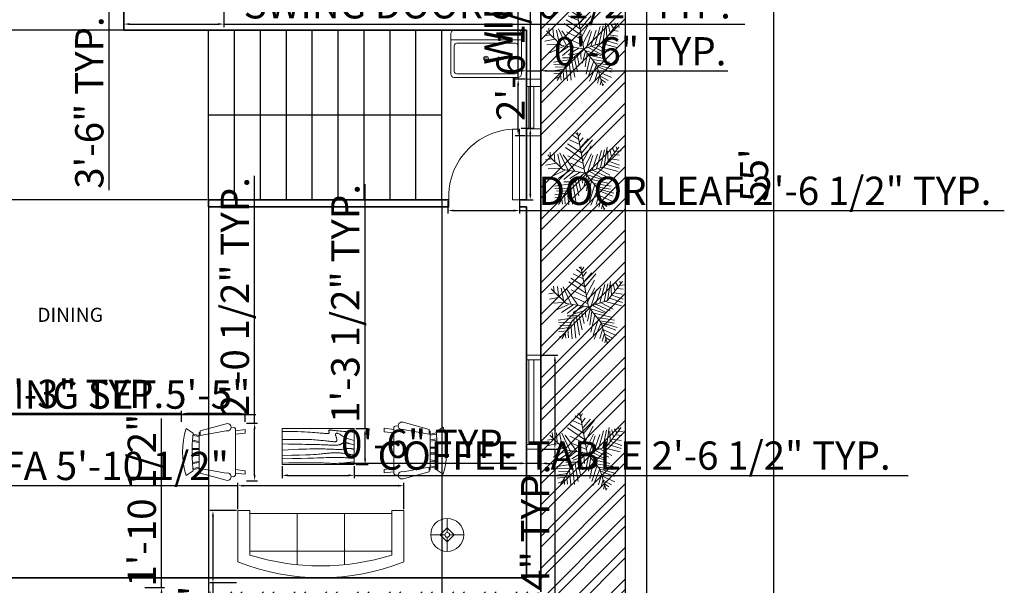
# Model space of a CAD drawing. Units: inches. Extents: x 2297 to 3143, y 440 to 1351.
# Tile 4 of 6: x 2725 to 3143, y 703 to 944. Entities that reach past the tile are written whole.
import ezdxf

# ---------------------------------------------------------------- set-up
doc = ezdxf.new("R2010")
doc.units = ezdxf.units.IN
for name, color, linetype, lineweight in [('A-ANNO-DIMS', 2, 'Continuous', 18), ('A-AREA-IDEN', 7, 'Continuous', 18), ('A-DOOR', 4, 'Continuous', 20), ('A-FLOR-FIXT', 9, 'Continuous', 18), ('A-FLOR-STRS', 7, 'Continuous', 25), ('A-FURN', 8, 'Continuous', 18), ('A-GLAZ', 4, 'Continuous', 18), ('A-WALL', 7, 'Continuous', 35), ('C-PROP', 7, 'Continuous', 25), ('C-SITE-PATT', 252, 'Continuous', 13), ('E-LITE', 9, 'Continuous', 13), ('L-PLNT', 3, 'Continuous', 13)]:
    doc.layers.add(name, color=color, linetype=linetype, lineweight=lineweight)
doc.styles.get("Standard").update_dxf_attribs({"font": 'arial.ttf'})
doc.dimstyles.new('ISO-25', dxfattribs={"dimtxt": 12, "dimasz": 2.5, "dimexe": 1.25, "dimexo": 0.625, "dimtad": 1, "dimdec": 1, "dimlunit": 3, "dimtxsty": 'Standard', "dimcen": 2.5, "dimadec": 0, "dimazin": 0, "dimtfac": 1, "dimtdec": 1, "dimtmove": 0, "dimatfit": 3, "dimfxl": 1, "dimarcsym": 0})

# ---------------------------------------------------------------- blocks, each defined once
blk = doc.blocks.new('Table - Rectangular Woodgrain 60 x 30 in.')
for p, q in [((0, 0), (0, -30)), ((60, 0), (0, 0)), ((60, -30), (60, 0)), ((0, -30), (60, -30))]:
    blk.add_line(p, q)
for points in [[(0, -2.4), (4.8155, -2.418), (9.0302, -2.4688), (12.709, -2.5477), (15.9167, -2.65), (18.7181, -2.7711), (21.1781, -2.9063), (23.3616, -3.0508), (25.3333, -3.2), (27.1477, -3.3495), (28.8172, -3.4958), (30.3437, -3.636), (31.7291, -3.7667), (32.9756, -3.8849), (34.0849, -3.9875), (35.059, -4.0714), (35.9, -4.1334), (36.6114, -4.1711), (37.2041, -4.1854), (37.6906, -4.1779), (38.0833, -4.15), (38.3948, -4.1034), (38.6375, -4.0396), (38.8239, -3.9602), (38.9666, -3.8667), (39.0764, -3.7608), (39.1573, -3.6448), (39.2116, -3.521), (39.2416, -3.3917), (39.2498, -3.2593), (39.2385, -3.1261), (39.21, -2.9944), (39.1666, -2.8667), (39.111, -2.7447), (39.0468, -2.6281), (38.978, -2.5163), (38.9083, -2.4083), (38.8418, -2.3035), (38.7823, -2.201), (38.7337, -2.1001), (38.7, -2), (38.6844, -1.9003), (38.6875, -1.8021), (38.7094, -1.707), (38.75, -1.6167), (38.8094, -1.5326), (38.8875, -1.4563), (38.9844, -1.3893), (39.1, -1.3333), (39.2351, -1.2896), (39.3937, -1.2583), (39.5804, -1.2396), (39.8, -1.2333), (40.057, -1.2396), (40.3562, -1.2583), (40.7023, -1.2896), (41.1, -1.3333), (41.5547, -1.3895), (42.0755, -1.4573), (42.6721, -1.5361), (43.3542, -1.625), (44.1316, -1.7233), (45.014, -1.8302), (46.0114, -1.9449), (47.1333, -2.0667), (48.3862, -2.1947), (49.7625, -2.3281), (51.2513, -2.4663), (52.8416, -2.6083), (54.5226, -2.7535), (56.2833, -2.9011), (58.1127, -3.0501), (60, -3.2)], [(0, -9.2), (6.5759, -9.0858), (11.9385, -9.0365), (16.2527, -9.0418), (19.6833, -9.0917), (22.3952, -9.1759), (24.5531, -9.2844), (26.322, -9.4069), (27.8666, -9.5333), (29.3241, -9.6553), (30.7203, -9.7719), (32.0532, -9.8837), (33.3208, -9.9917), (34.5213, -10.0965), (35.6526, -10.199), (36.7128, -10.2999), (37.7, -10.4), (38.6129, -10.4996), (39.4531, -10.5969), (40.223, -10.6895), (40.925, -10.775), (41.5613, -10.8512), (42.1344, -10.9156), (42.6465, -10.966), (43.1, -11), (43.4976, -11.0158), (43.8437, -11.0136), (44.143, -10.9942), (44.4, -10.9583), (44.6195, -10.9069), (44.8062, -10.8406), (44.9648, -10.7603), (45.1, -10.6667), (45.2155, -10.5598), (45.3114, -10.4365), (45.3871, -10.2929), (45.4416, -10.125), (45.4743, -9.929), (45.4844, -9.7011), (45.4709, -9.4371), (45.4333, -9.1333), (45.3716, -8.7883), (45.2896, -8.4104), (45.1919, -8.0107), (45.0833, -7.6), (44.9685, -7.1893), (44.8521, -6.7896), (44.7388, -6.4117), (44.6333, -6.0667), (44.54, -5.7628), (44.4614, -5.4979), (44.4001, -5.2675), (44.3583, -5.0667), (44.3384, -4.8909), (44.3427, -4.7354), (44.3736, -4.5956), (44.4333, -4.4667), (44.5236, -4.3453), (44.6427, -4.2333), (44.7884, -4.1339), (44.9583, -4.05), (45.1501, -3.9849), (45.3614, -3.9417), (45.59, -3.9234), (45.8333, -3.9333), (46.0915, -3.9749), (46.3734, -4.0531), (46.6906, -4.1736), (47.0542, -4.3417), (47.4756, -4.5629), (47.9661, -4.8427), (48.5372, -5.1866), (49.2, -5.6), (49.9676, -6.0844), (50.8594, -6.625), (51.8965, -7.2031), (53.1, -7.8), (54.491, -8.3969), (56.0906, -8.975), (57.9199, -9.5156), (60, -10)], [(0, -12.8), (5.1847, -12.9322), (9.6213, -13.0323), (13.3963, -13.1059), (16.5958, -13.1583), (19.3063, -13.1952), (21.614, -13.2219), (23.6054, -13.2439), (25.3666, -13.2667), (26.9728, -13.2947), (28.4531, -13.3281), (29.8256, -13.3663), (31.1083, -13.4083), (32.3191, -13.4535), (33.476, -13.501), (34.597, -13.5501), (35.7, -13.6), (36.7984, -13.6497), (37.8875, -13.6979), (38.9578, -13.743), (40, -13.7833), (41.0047, -13.8174), (41.9625, -13.8438), (42.864, -13.8607), (43.7, -13.8667), (44.4631, -13.8604), (45.1552, -13.8417), (45.7801, -13.8104), (46.3416, -13.7667), (46.8439, -13.7104), (47.2906, -13.6417), (47.6858, -13.5604), (48.0333, -13.4667), (48.3375, -13.3608), (48.6042, -13.2448), (48.8396, -13.121), (49.05, -12.9917), (49.2417, -12.8593), (49.4208, -12.7261), (49.5937, -12.5944), (49.7667, -12.4667), (49.9452, -12.3451), (50.1323, -12.2313), (50.3303, -12.1268), (50.5416, -12.0333), (50.7686, -11.9524), (51.0135, -11.8854), (51.2788, -11.8341), (51.5666, -11.8), (51.8785, -11.7843), (52.2116, -11.7865), (52.562, -11.8059), (52.926, -11.8417), (53.2998, -11.8931), (53.6795, -11.9594), (54.0614, -12.0397), (54.4416, -12.1333), (54.8223, -12.2401), (55.2293, -12.3625), (55.6942, -12.5037), (56.2489, -12.6667), (56.9251, -12.8547), (57.7545, -13.0708), (58.7689, -13.3182), (60, -13.6)], [(0, -18), (5.124, -17.7273), (9.6609, -17.5057), (13.6705, -17.3303), (17.2125, -17.1958), (20.3467, -17.0973), (23.1328, -17.0297), (25.6307, -16.9878), (27.9, -16.9667), (29.9928, -16.9617), (31.9302, -16.9703), (33.7254, -16.9907), (35.3917, -17.0208), (36.9423, -17.0588), (38.3906, -17.1026), (39.7499, -17.1503), (41.0333, -17.2), (42.2519, -17.2496), (43.4073, -17.2969), (44.4986, -17.3395), (45.525, -17.375), (46.4858, -17.4012), (47.3802, -17.4156), (48.2074, -17.416), (48.9667, -17.4), (49.6583, -17.3662), (50.2872, -17.3167), (50.8595, -17.2547), (51.3812, -17.1833), (51.8584, -17.1057), (52.2971, -17.025), (52.7034, -16.9443), (53.0833, -16.8667), (53.443, -16.7951), (53.789, -16.7313), (54.128, -16.6768), (54.4666, -16.6334), (54.8115, -16.6024), (55.1693, -16.5854), (55.5465, -16.5841), (55.95, -16.6), (56.3828, -16.6337), (56.8346, -16.6823), (57.2915, -16.7418), (57.7396, -16.8084), (58.165, -16.878), (58.5539, -16.9469), (58.8924, -17.0111), (59.1666, -17.0667), (59.3679, -17.1107), (59.5078, -17.1438), (59.6032, -17.1675), (59.6708, -17.1833), (59.7275, -17.193), (59.7901, -17.1979), (59.8753, -17.1998), (60, -17.2)], [(0, -22.4), (8.0098, -22.2501), (14.4094, -22.1011), (19.4168, -21.9535), (23.25, -21.8083), (26.1269, -21.6663), (28.2656, -21.5281), (29.884, -21.3947), (31.2, -21.2667), (32.3967, -21.1448), (33.5172, -21.0292), (34.5697, -20.9198), (35.5625, -20.8167), (36.5037, -20.7198), (37.4015, -20.6292), (38.2642, -20.5448), (39.1, -20.4667), (39.9164, -20.3951), (40.7187, -20.3313), (41.5117, -20.2768), (42.3, -20.2333), (43.0883, -20.2024), (43.8812, -20.1854), (44.6836, -20.1841), (45.5, -20.2), (46.3328, -20.234), (47.1747, -20.2844), (48.0163, -20.3488), (48.8479, -20.425), (49.66, -20.5106), (50.4429, -20.6031), (51.1872, -20.7004), (51.8833, -20.8), (52.5246, -20.8999), (53.1166, -20.9995), (53.6681, -21.0983), (54.1875, -21.1958), (54.6834, -21.2919), (55.1646, -21.3859), (55.6394, -21.4777), (56.1167, -21.5667), (56.6028, -21.6515), (57.0961, -21.7266), (57.5929, -21.7852), (58.0896, -21.8208), (58.5823, -21.8268), (59.0674, -21.7964), (59.5412, -21.723), (60, -21.6)], [(0, -25.2), (8.6355, -25.0504), (15.7026, -24.9031), (21.4049, -24.7606), (25.9458, -24.625), (29.529, -24.4988), (32.3578, -24.3844), (34.6359, -24.284), (36.5667, -24.2), (38.3213, -24.1341), (39.9417, -24.0854), (41.437, -24.0523), (42.8167, -24.0333), (44.0901, -24.0268), (45.2667, -24.0313), (46.3557, -24.0451), (47.3667, -24.0667), (48.309, -24.0947), (49.1928, -24.1287), (50.0284, -24.168), (50.826, -24.2125), (51.5959, -24.2617), (52.3483, -24.3151), (53.0935, -24.3725), (53.8417, -24.4334), (54.6009, -24.497), (55.3699, -24.561), (56.1454, -24.6226), (56.9239, -24.6792), (57.7021, -24.7279), (58.4764, -24.7662), (59.2435, -24.7911), (60, -24.8)], [(0, -28.8), (5.6867, -28.6681), (10.45, -28.5698), (14.407, -28.5012), (17.675, -28.4584), (20.3711, -28.4374), (22.6125, -28.4344), (24.5164, -28.4455), (26.2, -28.4667), (27.762, -28.4947), (29.2276, -28.5281), (30.6033, -28.5663), (31.8958, -28.6084), (33.1118, -28.6535), (34.2578, -28.7011), (35.3405, -28.7501), (36.3666, -28.8), (37.3443, -28.8497), (38.288, -28.8974), (39.2137, -28.9412), (40.1375, -28.9792), (41.0753, -29.0093), (42.0432, -29.0297), (43.0572, -29.0384), (44.1333, -29.0333), (45.2936, -29.0114), (46.5843, -28.9641), (48.0579, -28.8816), (49.7666, -28.7542), (51.7629, -28.5721), (54.0989, -28.3255), (56.8272, -28.0048), (60, -27.6)]]:
    blk.add_lwpolyline(points)
blk = doc.blocks.new('Sofa - Roundback 7 ft.')
for p, q in [((-12.00002, -32.4421), (-12.00003, -6.5971)), ((11.99997, -32.4421), (11.99998, -6.5971)), ((-36.000027, -34), (-36.000027, -11.4696)), ((-35.999844, -13.3819), (35.9998, -13.3819)), ((35.99998, -34), (35.99998, -11.4696)), ((-36.000027, -32.4421), (35.99998, -32.4421))]:
    blk.add_line(p, q)
for points in [[(-36.000027, -34), (-42.000027, -34), (-42.000027, -8)], [(41.99998, -8), (41.99998, -34), (35.99998, -34)]]:
    blk.add_lwpolyline(points)
for centre, radius, start, end in [((0, -114.25), 114.25, 68.43141, 111.5686), ((-0.00001, -127.1968), 121.1968, 72.72033, 107.2797)]:
    blk.add_arc(centre, radius, start, end)
blk = doc.blocks.new('Chair - Rocking')
for p, q in [((-8, -4.5), (-10, -1.5)), ((-4, -7), (-4.40532, -4.16272)), ((-1.5, -4.05012), (-1.5, -7)), ((-1, -7), (-1, -4.05012)), ((1, -7), (1, -4.04655)), ((1.5, -4.05012), (1.5, -7)), ((8, -4.5), (10, -1.5)), ((-9, -7.5), (-12, -18.49999)), ((-7, -7.5), (-9, -7.5)), ((-9, -18.49999), (-7, -7.5)), ((-8.23428, -6.99939), (-8.3093, -7.47958)), ((-8.23041, -7), (8.23915, -7)), ((-7.5, -4.5), (-7, -7)), ((-6.5, -7), (-7.02225, -4.43)), ((-4.5, -7), (-4.96674, -4.19951)), ((4, -7), (4.40187, -4.18694)), ((4.5, -7), (4.96761, -4.19437)), ((6.5, -7), (7, -4.4057)), ((7.5, -4.5), (7, -7)), ((7, -7.5), (9, -7.5)), ((9, -18.49999), (7, -7.5)), ((8.31071, -7.48854), (8.23449, -7.00073)), ((9, -7.5), (12, -18.49999)), ((-10.36644, -20.64523), (-10.5, -21.49999)), ((10.5, -21.49999), (10.3575, -20.58798)), ((-9, -22.49999), (-9.5, -26.49999)), ((0, -22.49999), (-9.5, -22.49999)), ((-8, -26.49999), (-7.5, -22.49999)), ((0, -22.49999), (9.5, -22.49999)), ((8, -26.49999), (7.5, -22.49999)), ((9, -22.49999), (9.5, -26.49999)), ((-9.5, -26.49999), (-8, -26.49999)), ((9.5, -26.49999), (8, -26.49999))]:
    blk.add_line(p, q)
for centre, radius, start, end in [((0, -34.08333), 34.08333, 72.93847, 107.0615), ((0, -68.25004), 64.25, 93.92211, 97.15267), ((0, -68.25004), 64.25, 82.84733, 93.92211), ((-10.5, -18.99999), 1.58114, 161.5651, 18.43495), ((10.5, -18.99999), 1.58114, 161.5651, 18.43495), ((-9.5, -21.49999), 1, 180, 270), ((9.5, -21.49999), 1, 270, 0)]:
    blk.add_arc(centre, radius, start, end)
blk = doc.blocks.new('Sink-single - 30 in top')
blk.add_line((-15, -3.999996), (15, -3.999996))
for points in [[(-13.5, 0), (13.5, 0)], [(-15, -18.499996), (-15, -1.5)], [(15, -1.5), (15, -18.499996)], [(-13.5, -17.499996), (-13.5, -6.499996)], [(-12.5, -5.499996), (12.5, -5.499996)], [(13.5, -6.499996), (13.5, -17.499996)], [(13.5, -19.999996), (-13.5, -19.999996)], [(12.5, -18.499996), (-12.5, -18.499996)]]:
    blk.add_lwpolyline(points)
for radius in [1, 0.5]:
    blk.add_circle((0, -11.999996), radius)
for centre, radius, start, end in [((-13.5, -1.5), 1.5, 90, 180), ((13.5, -1.5), 1.5, 0, 90), ((-12.5, -6.499996), 1, 90, 180), ((12.5, -6.499996), 1, 0, 90), ((-13.5, -18.499996), 1.5, 180, 270), ((-12.5, -17.499996), 1, 180, 270), ((12.5, -17.499996), 1, 270, 0), ((13.5, -18.499996), 1.5, 270, 0)]:
    blk.add_arc(centre, radius, start, end)
blk = doc.blocks.new('*U16')
for p, q in [((-10.186, 53.64), (-13.084, 55.962)), ((0, 0), (-10.5, 57)), ((-9.099, 51.782), (-6.563, 55.962)), ((-7.288, 39.707), (-21.778, 46.673)), ((-8.737, 47.138), (-17.069, 52.711)), ((-7.65, 43.423), (-2.578, 49.46)), ((-5.839, 35.992), (4.667, 48.067)), ((-5.114, 27.632), (10.463, 46.673)), ((-48.585, 21.131), (-49.309, 29.026)), ((-43.513, 28.561), (-42.427, 15.558)), ((-35.544, 28.097), (-24.314, 3.947)), ((-3.665, 19.273), (-27.574, 35.527)), ((-5.114, 28.097), (-24.676, 40.636)), ((-2.941, 16.486), (8.652, 37.85)), ((16.259, 5.805), (23.142, 31.348)), ((22.055, 7.198), (27.489, 32.277)), ((27, 9), (48, 36)), ((27.127, 9.056), (31.112, 35.992)), ((31.836, 30.883), (32.561, 16.486)), ((35.096, 32.741), (37.27, 22.524)), ((38.719, 34.134), (41.979, 28.561)), ((43.791, 29.954), (51.036, 30.883)), ((44.153, 36.456), (45.239, 32.741)), ((-47.498, 19.737), (-55.83, 18.344)), ((-31.5, 4.5), (-52.5, 25.5)), ((-38.442, 26.239), (-34.819, 7.663)), ((-14.533, 2.09), (-30.834, 25.31)), ((-24.314, 23.917), (-2.941, 13.7)), ((-1.129, 6.734), (9.014, 26.704)), ((3.942, 1.625), (11.187, 24.381)), ((10.101, 3.483), (17.708, 26.239)), ((33.285, 16.486), (48.862, 10.913)), ((36.183, 19.737), (48.137, 17.88)), ((40.53, 25.775), (48.862, 24.846)), ((-40.615, 13.7), (-55.105, 10.913)), ((-33.37, 6.269), (-52.207, 5.34)), ((-28.299, 3.483), (-47.86, -5.805)), ((-21.416, 3.018), (-38.079, -8.128)), ((0, 0), (-31.5, 4.5)), ((-15.982, 2.09), (-30.11, -9.521)), ((0, 0), (-22.5, -19.5)), ((-6.563, 1.161), (-21.416, -8.128)), ((-20.691, 13.7), (-1.129, 4.876)), ((0, 0), (27, 9)), ((0, 0), (18, -22.5)), ((6.478, 1.625), (26.04, -8.592)), ((11.187, 3.483), (30.749, -5.805)), ((18.07, 5.805), (35.096, -3.483)), ((24.229, 7.663), (46.688, 1.625)), ((29.662, 12.307), (48.137, 6.269)), ((-15.257, -12.772), (-30.11, -12.772)), ((-6.563, -5.805), (-19.967, -9.985)), ((-13.446, -11.378), (-8.737, -32.741)), ((-9.461, -8.592), (-6.201, -23.453)), ((-4.752, -3.483), (-3.665, -14.629)), ((2.493, -3.019), (-1.491, -20.202)), ((1.769, -2.555), (24.229, -9.521)), ((5.029, -6.27), (2.131, -25.775)), ((9.014, -11.378), (3.58, -35.992)), ((7.565, -9.056), (32.198, -14.629)), ((-17.431, -15.094), (-42.789, -18.809)), ((-24.314, -21.596), (-42.427, -22.06)), ((-26.849, -26.24), (-40.253, -25.775)), ((-22.5, -19.5), (-37.5, -45)), ((-25.038, -23.918), (-22.865, -45.281)), ((-20.691, -18.345), (-17.793, -44.352)), ((-17.069, -15.094), (-12.721, -40.172)), ((14.085, -16.951), (6.478, -40.172)), ((18.07, -22.524), (8.289, -45.745)), ((12.274, -15.094), (36.907, -18.809)), ((16.259, -19.738), (36.183, -22.989)), ((18, -22.5), (27, -52.5)), ((18.433, -22.524), (40.53, -29.026)), ((19.157, -25.311), (38.719, -33.206)), ((-28.299, -29.026), (-42.789, -31.348)), ((-30.834, -34.135), (-42.427, -35.528)), ((-34.457, -39.708), (-40.978, -42.494)), ((-32.646, -36.921), (-31.921, -44.352)), ((-29.023, -30.884), (-27.936, -43.887)), ((20.244, -30.419), (15.897, -44.816)), ((22.78, -37.85), (19.519, -48.532)), ((21.331, -32.741), (39.081, -40.636)), ((22.78, -38.314), (34.372, -44.816)), ((24.591, -45.745), (23.142, -50.854)), ((24.591, -43.423), (30.749, -47.603)), ((26.764, -49.925), (28.213, -50.854))]:
    blk.add_line(p, q)
blk = doc.blocks.new('*D18')
at = {"layer": 'A-ANNO-DIMS', "color": 0, "lineweight": -2, "transparency": 16777216}
for p, q in [((2993.8, 1207.63), (3046.74, 1207.63)), ((3045.49, 1205.13), (3045.49, 550.13)), ((2992.32, 547.63), (3046.74, 547.63))]:
    blk.add_line(p, q, dxfattribs=at)
at = {"layer": 'A-ANNO-DIMS', "color": 0, "transparency": 16777216}
for points in [[(3045.07, 1205.13), (3045.91, 1205.13), (3045.49, 1207.63)], [(3045.07, 550.13), (3045.91, 550.13), (3045.49, 547.63)]]:
    blk.add_solid(points, dxfattribs=at)
at = {"layer": 'Defpoints', "color": 0, "transparency": 16777216}
for p in [(2993.18, 1207.63), (2991.69, 547.63), (3045.49, 547.63)]:
    blk.add_point(p, dxfattribs=at)
at = {"layer": 'A-ANNO-DIMS', "color": 0, "transparency": 16777216, "insert": (3038.76, 877.63), "char_height": 12, "attachment_point": 5, "rotation": 90}
blk.add_mtext("55'", dxfattribs=at)
blk = doc.blocks.new('Lamp - Table')
for p, q in [((0, 7), (0, 1)), ((-1, 0), (-7, 0)), ((0, 3), (-3, 0)), ((-3, 0), (0, -3)), ((3, 0), (0, 3)), ((0, -3), (3, 0)), ((1, 0), (7, 0)), ((0, -1), (0, -7))]:
    blk.add_line(p, q)
for radius in [7, 1]:
    blk.add_circle((0, 0), radius)
blk = doc.blocks.new('DOOR-30IN-LEAF')
blk.add_lwpolyline([(30, 0), (27, 0), (27, 30), (30, 30)], close=True)
blk.add_arc((28.5, 1.5), 28.54, 86.9872, 183.0128)
blk = doc.blocks.new('WIN-36IN-6IN-WALL')
for p, q in [((6, 40), (0, 40)), ((6, 38), (0, 38)), ((3, 38), (3, 2)), ((5, 38), (5, 2)), ((0, 2), (6, 2)), ((0, 0), (6, 0))]:
    blk.add_line(p, q)
blk = doc.blocks.new('WIN-18IN-6IN-WALL')
for p, q in [((6, 24), (0, 24)), ((6, 21), (0, 21)), ((1, 3), (1, 21)), ((3, 3), (3, 21)), ((0, 3), (6, 3)), ((0, 0), (6, 0))]:
    blk.add_line(p, q)
blk = doc.blocks.new('*D29')
at = {"layer": 'A-ANNO-DIMS', "color": 0, "lineweight": -2, "transparency": 16777216}
for p, q in [((2769.69, 947.51), (2769.69, 940.52)), ((2812.11, 947.51), (2812.11, 940.52)), ((2772.19, 941.77), (2809.61, 941.77)), ((2812.11, 941.77), (3033.33, 941.77))]:
    blk.add_line(p, q, dxfattribs=at)
at = {"layer": 'A-ANNO-DIMS', "color": 0, "transparency": 16777216}
for points in [[(2772.19, 942.19), (2772.19, 941.35), (2769.69, 941.77)], [(2809.61, 942.19), (2809.61, 941.35), (2812.11, 941.77)]]:
    blk.add_solid(points, dxfattribs=at)
at = {"layer": 'Defpoints', "color": 0, "transparency": 16777216}
for p in [(2769.69, 948.13), (2812.11, 948.13), (2812.11, 941.77)]:
    blk.add_point(p, dxfattribs=at)
at = {"layer": 'A-ANNO-DIMS', "color": 0, "transparency": 16777216, "insert": (2923.97, 948.61), "char_height": 12, "attachment_point": 5}
blk.add_mtext('SWING DOOR 3\'-6 1/2" TYP.', dxfattribs=at)
blk = doc.blocks.new('*D30')
at = {"layer": 'A-ANNO-DIMS', "color": 0, "lineweight": -2, "transparency": 16777216}
for p, q in [((2769.07, 990.13), (2762.08, 990.13)), ((2763.33, 987.63), (2763.33, 950.63)), ((2769.07, 948.13), (2762.08, 948.13)), ((2763.33, 948.13), (2763.33, 871.25))]:
    blk.add_line(p, q, dxfattribs=at)
at = {"layer": 'A-ANNO-DIMS', "color": 0, "transparency": 16777216}
for points in [[(2762.91, 987.63), (2763.75, 987.63), (2763.33, 990.13)], [(2762.91, 950.63), (2763.75, 950.63), (2763.33, 948.13)]]:
    blk.add_solid(points, dxfattribs=at)
at = {"layer": 'Defpoints', "color": 0, "transparency": 16777216}
for p in [(2769.69, 990.13), (2763.33, 948.13), (2769.69, 948.13)]:
    blk.add_point(p, dxfattribs=at)
at = {"layer": 'A-ANNO-DIMS', "color": 0, "transparency": 16777216, "insert": (2756.57, 908.44), "char_height": 12, "attachment_point": 5, "rotation": 90}
blk.add_mtext('3\'-6" TYP.', dxfattribs=at)
blk = doc.blocks.new('*D31')
at = {"layer": 'A-ANNO-DIMS', "color": 0, "lineweight": -2, "transparency": 16777216}
for p, q in [((2947.32, 801.2), (2953.94, 801.2)), ((2952.69, 798.7), (2952.69, 763.7)), ((2947.32, 761.2), (2953.94, 761.2)), ((2952.69, 761.2), (2952.69, 605.6))]:
    blk.add_line(p, q, dxfattribs=at)
at = {"layer": 'A-ANNO-DIMS', "color": 0, "transparency": 16777216}
for points in [[(2952.28, 798.7), (2953.11, 798.7), (2952.69, 801.2)], [(2952.28, 763.7), (2953.11, 763.7), (2952.69, 761.2)]]:
    blk.add_solid(points, dxfattribs=at)
at = {"layer": 'Defpoints', "color": 0, "transparency": 16777216}
for p in [(2946.69, 801.2), (2946.69, 761.2), (2952.69, 761.2)]:
    blk.add_point(p, dxfattribs=at)
at = {"layer": 'A-ANNO-DIMS', "color": 0, "transparency": 16777216, "insert": (2945.85, 682.15), "char_height": 12, "attachment_point": 5, "rotation": 90}
blk.add_mtext('WINDOW 3\'-4" TYP.', dxfattribs=at)
blk = doc.blocks.new('*D32')
at = {"layer": 'A-ANNO-DIMS', "color": 0, "lineweight": -2, "transparency": 16777216}
for p, q in [((2940.69, 760.58), (2940.69, 753.95)), ((2946.69, 760.58), (2946.69, 753.95)), ((2938.19, 755.2), (2861.3, 755.2)), ((2946.69, 755.2), (2940.69, 755.2)), ((2949.19, 755.2), (2951.69, 755.2))]:
    blk.add_line(p, q, dxfattribs=at)
at = {"layer": 'A-ANNO-DIMS', "color": 0, "transparency": 16777216}
for points in [[(2938.19, 755.62), (2938.19, 754.78), (2940.69, 755.2)], [(2949.19, 755.62), (2949.19, 754.78), (2946.69, 755.2)]]:
    blk.add_solid(points, dxfattribs=at)
at = {"layer": 'Defpoints', "color": 0, "transparency": 16777216}
for p in [(2940.69, 761.2), (2946.69, 761.2), (2940.69, 755.2)]:
    blk.add_point(p, dxfattribs=at)
at = {"layer": 'A-ANNO-DIMS', "color": 0, "transparency": 16777216, "insert": (2898.49, 761.95), "char_height": 12, "attachment_point": 5}
blk.add_mtext('0\'-6" TYP.', dxfattribs=at)
blk = doc.blocks.new('*D43')
at = {"layer": 'A-ANNO-DIMS', "color": 0, "lineweight": -2, "transparency": 16777216}
for p, q in [((2937.09, 918.32), (2937.09, 1073.92)), ((2940.07, 918.32), (2935.84, 918.32)), ((2937.09, 896.82), (2937.09, 915.82)), ((2940.07, 894.32), (2935.84, 894.32))]:
    blk.add_line(p, q, dxfattribs=at)
at = {"layer": 'A-ANNO-DIMS', "color": 0, "transparency": 16777216}
for points in [[(2936.68, 915.82), (2937.51, 915.82), (2937.09, 918.32)], [(2936.68, 896.82), (2937.51, 896.82), (2937.09, 894.32)]]:
    blk.add_solid(points, dxfattribs=at)
at = {"layer": 'Defpoints', "color": 0, "transparency": 16777216}
for p in [(2937.09, 918.32), (2940.69, 918.32), (2940.69, 894.32)]:
    blk.add_point(p, dxfattribs=at)
at = {"layer": 'A-ANNO-DIMS', "color": 0, "transparency": 16777216, "insert": (2930.26, 997.37), "char_height": 12, "attachment_point": 5, "rotation": 90}
blk.add_mtext('WINDOW 2\'-0" TYP.', dxfattribs=at)
blk = doc.blocks.new('*D44')
at = {"layer": 'A-ANNO-DIMS', "color": 0, "lineweight": -2, "transparency": 16777216}
for p, q in [((2938.19, 921.92), (2935.69, 921.92)), ((2940.69, 918.95), (2940.69, 923.17)), ((2940.69, 921.92), (2946.69, 921.92)), ((2946.69, 918.95), (2946.69, 923.17)), ((2949.19, 921.92), (3026.09, 921.92))]:
    blk.add_line(p, q, dxfattribs=at)
at = {"layer": 'A-ANNO-DIMS', "color": 0, "transparency": 16777216}
for points in [[(2938.19, 922.34), (2938.19, 921.5), (2940.69, 921.92)], [(2949.19, 922.34), (2949.19, 921.5), (2946.69, 921.92)]]:
    blk.add_solid(points, dxfattribs=at)
at = {"layer": 'Defpoints', "color": 0, "transparency": 16777216}
for p in [(2946.69, 921.92), (2940.69, 918.32), (2946.69, 918.32)]:
    blk.add_point(p, dxfattribs=at)
at = {"layer": 'A-ANNO-DIMS', "color": 0, "transparency": 16777216, "insert": (2988.89, 928.67), "char_height": 12, "attachment_point": 5}
blk.add_mtext('0\'-6" TYP.', dxfattribs=at)
blk = doc.blocks.new('*D45')
at = {"layer": 'A-ANNO-DIMS', "color": 0, "lineweight": -2, "transparency": 16777216}
for p, q in [((2836.9, 754.07), (2836.9, 748.85)), ((2867.52, 754.07), (2867.52, 748.85)), ((2839.4, 750.1), (2865.02, 750.1)), ((2867.52, 750.1), (3102.65, 750.1))]:
    blk.add_line(p, q, dxfattribs=at)
at = {"layer": 'A-ANNO-DIMS', "color": 0, "transparency": 16777216}
for points in [[(2839.4, 750.52), (2839.4, 749.69), (2836.9, 750.1)], [(2865.02, 750.52), (2865.02, 749.69), (2867.52, 750.1)]]:
    blk.add_solid(points, dxfattribs=at)
at = {"layer": 'Defpoints', "color": 0, "transparency": 16777216}
for p in [(2836.9, 754.69), (2867.52, 754.69), (2867.52, 750.1)]:
    blk.add_point(p, dxfattribs=at)
at = {"layer": 'A-ANNO-DIMS', "color": 0, "transparency": 16777216, "insert": (2986.33, 756.94), "char_height": 12, "attachment_point": 5}
blk.add_mtext('COFFEE TABLE 2\'-6 1/2" TYP.', dxfattribs=at)
blk = doc.blocks.new('*D46')
at = {"layer": 'A-ANNO-DIMS', "color": 0, "lineweight": -2, "transparency": 16777216}
for p, q in [((2872.11, 770), (2872.11, 873.73)), ((2868.14, 770), (2873.36, 770)), ((2872.11, 757.19), (2872.11, 767.5)), ((2868.14, 754.69), (2873.36, 754.69))]:
    blk.add_line(p, q, dxfattribs=at)
at = {"layer": 'A-ANNO-DIMS', "color": 0, "transparency": 16777216}
for points in [[(2871.69, 767.5), (2872.53, 767.5), (2872.11, 770)], [(2871.69, 757.19), (2872.53, 757.19), (2872.11, 754.69)]]:
    blk.add_solid(points, dxfattribs=at)
at = {"layer": 'Defpoints', "color": 0, "transparency": 16777216}
for p in [(2867.52, 770), (2872.11, 770), (2867.52, 754.69)]:
    blk.add_point(p, dxfattribs=at)
at = {"layer": 'A-ANNO-DIMS', "color": 0, "transparency": 16777216, "insert": (2865.27, 823.11), "char_height": 12, "attachment_point": 5, "rotation": 90}
blk.add_mtext('1\'-3 1/2" TYP.', dxfattribs=at)
blk = doc.blocks.new('*D48')
at = {"layer": 'A-ANNO-DIMS', "color": 0, "lineweight": -2, "transparency": 16777216}
for p, q in [((2778.39, 676.96), (2778.39, 683.36)), ((2780.89, 682.11), (2799.4, 682.11)), ((2801.9, 676.96), (2801.9, 683.36)), ((2801.9, 682.11), (2914.95, 682.11))]:
    blk.add_line(p, q, dxfattribs=at)
at = {"layer": 'A-ANNO-DIMS', "color": 0, "transparency": 16777216}
for points in [[(2780.89, 682.52), (2780.89, 681.69), (2778.39, 682.11)], [(2799.4, 682.52), (2799.4, 681.69), (2801.9, 682.11)]]:
    blk.add_solid(points, dxfattribs=at)
at = {"layer": 'Defpoints', "color": 0, "transparency": 16777216}
for p in [(2801.9, 682.11), (2778.39, 676.34), (2801.9, 676.34)]:
    blk.add_point(p, dxfattribs=at)
at = {"layer": 'A-ANNO-DIMS', "color": 0, "transparency": 16777216, "insert": (2859.68, 688.94), "char_height": 12, "attachment_point": 5}
blk.add_mtext('1\'-11 1/2" TYP.', dxfattribs=at)
blk = doc.blocks.new('*D49')
at = {"layer": 'A-ANNO-DIMS', "color": 0, "lineweight": -2, "transparency": 16777216}
for p, q in [((2818.08, 745.72), (2694.9, 745.72)), ((2818.08, 735.78), (2818.08, 746.97)), ((2886.03, 745.72), (2820.58, 745.72)), ((2888.53, 735.78), (2888.53, 746.97))]:
    blk.add_line(p, q, dxfattribs=at)
at = {"layer": 'A-ANNO-DIMS', "color": 0, "transparency": 16777216}
for points in [[(2820.58, 746.14), (2820.58, 745.3), (2818.08, 745.72)], [(2886.03, 746.14), (2886.03, 745.3), (2888.53, 745.72)]]:
    blk.add_solid(points, dxfattribs=at)
at = {"layer": 'Defpoints', "color": 0, "transparency": 16777216}
for p in [(2818.08, 745.72), (2818.08, 735.15), (2888.53, 735.15)]:
    blk.add_point(p, dxfattribs=at)
at = {"layer": 'A-ANNO-DIMS', "color": 0, "transparency": 16777216, "insert": (2755.24, 752.55), "char_height": 12, "attachment_point": 5}
blk.add_mtext('SOFA 5\'-10 1/2"', dxfattribs=at)
blk = doc.blocks.new('*D50')
at = {"layer": 'A-ANNO-DIMS', "color": 0, "lineweight": -2, "transparency": 16777216}
for p, q in [((2817.45, 735.15), (2806.26, 735.15)), ((2807.51, 732.65), (2807.51, 706.9)), ((2817.45, 704.4), (2806.26, 704.4)), ((2807.51, 704.4), (2807.51, 668.54))]:
    blk.add_line(p, q, dxfattribs=at)
at = {"layer": 'A-ANNO-DIMS', "color": 0, "transparency": 16777216}
for points in [[(2807.09, 732.65), (2807.92, 732.65), (2807.51, 735.15)], [(2807.09, 706.9), (2807.92, 706.9), (2807.51, 704.4)]]:
    blk.add_solid(points, dxfattribs=at)
at = {"layer": 'Defpoints', "color": 0, "transparency": 16777216}
for p in [(2818.08, 735.15), (2807.51, 704.4), (2818.08, 704.4)]:
    blk.add_point(p, dxfattribs=at)
at = {"layer": 'A-ANNO-DIMS', "color": 0, "transparency": 16777216, "insert": (2800.86, 685.22), "char_height": 12, "attachment_point": 5, "rotation": 90}
blk.add_mtext('2\'-7"', dxfattribs=at)
blk = doc.blocks.new('*D52')
at = {"layer": 'A-ANNO-DIMS', "color": 0, "lineweight": -2, "transparency": 16777216}
for p, q in [((2785.68, 702.41), (2785.68, 774.21)), ((2778.53, 702.41), (2786.93, 702.41)), ((2785.68, 682.29), (2785.68, 699.91)), ((2778.53, 679.79), (2786.93, 679.79))]:
    blk.add_line(p, q, dxfattribs=at)
at = {"layer": 'A-ANNO-DIMS', "color": 0, "transparency": 16777216}
for points in [[(2785.26, 699.91), (2786.09, 699.91), (2785.68, 702.41)], [(2785.26, 682.29), (2786.09, 682.29), (2785.68, 679.79)]]:
    blk.add_solid(points, dxfattribs=at)
at = {"layer": 'Defpoints', "color": 0, "transparency": 16777216}
for p in [(2777.91, 702.41), (2785.68, 702.41), (2777.91, 679.79)]:
    blk.add_point(p, dxfattribs=at)
at = {"layer": 'A-ANNO-DIMS', "color": 0, "transparency": 16777216, "insert": (2778.85, 739.56), "char_height": 12, "attachment_point": 5, "rotation": 90}
blk.add_mtext('1\'-10 1/2"', dxfattribs=at)
blk = doc.blocks.new('*D53')
at = {"layer": 'A-ANNO-DIMS', "color": 0, "lineweight": -2, "transparency": 16777216}
for p, q in [((2794.15, 772.88), (2794.15, 777.56)), ((2821.15, 772.88), (2821.15, 777.56)), ((2794.15, 776.31), (2641.5, 776.31)), ((2818.65, 776.31), (2796.65, 776.31))]:
    blk.add_line(p, q, dxfattribs=at)
at = {"layer": 'A-ANNO-DIMS', "color": 0, "transparency": 16777216}
for points in [[(2796.65, 776.72), (2796.65, 775.89), (2794.15, 776.31)], [(2818.65, 776.72), (2818.65, 775.89), (2821.15, 776.31)]]:
    blk.add_solid(points, dxfattribs=at)
at = {"layer": 'Defpoints', "color": 0, "transparency": 16777216}
for p in [(2794.15, 776.31), (2794.15, 772.26), (2821.15, 772.26)]:
    blk.add_point(p, dxfattribs=at)
at = {"layer": 'A-ANNO-DIMS', "color": 0, "transparency": 16777216, "insert": (2716.58, 783.14), "char_height": 12, "attachment_point": 5}
blk.add_mtext('ROCKER 2\'-3" TYP.', dxfattribs=at)
blk = doc.blocks.new('*D54')
at = {"layer": 'A-ANNO-DIMS', "color": 0, "lineweight": -2, "transparency": 16777216}
for p, q in [((2825.2, 772.26), (2825.2, 877.32)), ((2821.78, 772.26), (2826.45, 772.26)), ((2825.2, 750.32), (2825.2, 769.76)), ((2821.78, 747.82), (2826.45, 747.82))]:
    blk.add_line(p, q, dxfattribs=at)
at = {"layer": 'A-ANNO-DIMS', "color": 0, "transparency": 16777216}
for points in [[(2824.79, 769.76), (2825.62, 769.76), (2825.2, 772.26)], [(2824.79, 750.32), (2825.62, 750.32), (2825.2, 747.82)]]:
    blk.add_solid(points, dxfattribs=at)
at = {"layer": 'Defpoints', "color": 0, "transparency": 16777216}
for p in [(2821.15, 772.26), (2825.2, 772.26), (2821.15, 747.82)]:
    blk.add_point(p, dxfattribs=at)
at = {"layer": 'A-ANNO-DIMS', "color": 0, "transparency": 16777216, "insert": (2818.37, 826.04), "char_height": 12, "attachment_point": 5, "rotation": 90}
blk.add_mtext('2\'-0 1/2" TYP.', dxfattribs=at)
blk = doc.blocks.new('*D57')
at = {"layer": 'A-ANNO-DIMS', "color": 0, "lineweight": -2, "transparency": 16777216}
for p, q in [((2907.27, 866.51), (2907.27, 861.32)), ((2937.69, 866.51), (2937.69, 861.32)), ((2909.77, 862.57), (2935.19, 862.57)), ((2937.69, 862.57), (3143.49, 862.57))]:
    blk.add_line(p, q, dxfattribs=at)
at = {"layer": 'A-ANNO-DIMS', "color": 0, "transparency": 16777216}
for points in [[(2909.77, 862.99), (2909.77, 862.15), (2907.27, 862.57)], [(2935.19, 862.99), (2935.19, 862.15), (2937.69, 862.57)]]:
    blk.add_solid(points, dxfattribs=at)
at = {"layer": 'Defpoints', "color": 0, "transparency": 16777216}
for p in [(2907.27, 867.13), (2937.69, 867.13), (2937.69, 862.57)]:
    blk.add_point(p, dxfattribs=at)
at = {"layer": 'A-ANNO-DIMS', "color": 0, "transparency": 16777216, "insert": (3041.84, 869.4), "char_height": 12, "attachment_point": 5}
blk.add_mtext('DOOR LEAF 2\'-6 1/2" TYP.', dxfattribs=at)
blk = doc.blocks.new('*D58')
at = {"layer": 'A-ANNO-DIMS', "color": 0, "lineweight": -2, "transparency": 16777216}
for p, q in [((2942.26, 897.56), (2942.26, 1002.62)), ((2938.32, 897.56), (2943.51, 897.56)), ((2942.26, 869.63), (2942.26, 895.06)), ((2938.32, 867.13), (2943.51, 867.13))]:
    blk.add_line(p, q, dxfattribs=at)
at = {"layer": 'A-ANNO-DIMS', "color": 0, "transparency": 16777216}
for points in [[(2941.84, 895.06), (2942.67, 895.06), (2942.26, 897.56)], [(2941.84, 869.63), (2942.67, 869.63), (2942.26, 867.13)]]:
    blk.add_solid(points, dxfattribs=at)
at = {"layer": 'Defpoints', "color": 0, "transparency": 16777216}
for p in [(2937.69, 897.56), (2942.26, 897.56), (2937.69, 867.13)]:
    blk.add_point(p, dxfattribs=at)
at = {"layer": 'A-ANNO-DIMS', "color": 0, "transparency": 16777216, "insert": (2935.43, 951.34), "char_height": 12, "attachment_point": 5, "rotation": 90}
blk.add_mtext('2\'-6 1/2" TYP.', dxfattribs=at)
blk = doc.blocks.new('*D63')
at = {"layer": 'A-ANNO-DIMS', "color": 0, "lineweight": -2, "transparency": 16777216}
for p, q in [((2625.28, 785.11), (2625.28, 774.77)), ((2690.07, 785.11), (2690.07, 774.77)), ((2627.78, 776.02), (2687.57, 776.02)), ((2690.07, 776.02), (2825.72, 776.02))]:
    blk.add_line(p, q, dxfattribs=at)
at = {"layer": 'A-ANNO-DIMS', "color": 0, "transparency": 16777216}
for points in [[(2627.78, 776.44), (2627.78, 775.6), (2625.28, 776.02)], [(2687.57, 776.44), (2687.57, 775.6), (2690.07, 776.02)]]:
    blk.add_solid(points, dxfattribs=at)
at = {"layer": 'Defpoints', "color": 0, "transparency": 16777216}
for p in [(2625.28, 785.74), (2690.07, 785.74), (2690.07, 776.02)]:
    blk.add_point(p, dxfattribs=at)
at = {"layer": 'A-ANNO-DIMS', "color": 0, "transparency": 16777216, "insert": (2759.14, 782.85), "char_height": 12, "attachment_point": 5}
blk.add_mtext('DINING SET 5\'-5"', dxfattribs=at)
blk = doc.blocks.new('*D79')
at = {"layer": 'A-ANNO-DIMS', "color": 0, "lineweight": -2, "transparency": 16777216}
for p, q in [((2805.69, 866.51), (2805.69, 510.33)), ((2904.69, 866.51), (2904.69, 510.33)), ((2808.19, 511.58), (2902.19, 511.58))]:
    blk.add_line(p, q, dxfattribs=at)
at = {"layer": 'A-ANNO-DIMS', "color": 0, "transparency": 16777216}
for points in [[(2808.19, 512), (2808.19, 511.17), (2805.69, 511.58)], [(2902.19, 512), (2902.19, 511.17), (2904.69, 511.58)]]:
    blk.add_solid(points, dxfattribs=at)
at = {"layer": 'Defpoints', "color": 0, "transparency": 16777216}
for p in [(2805.69, 867.13), (2904.69, 867.13), (2904.69, 511.58)]:
    blk.add_point(p, dxfattribs=at)
at = {"layer": 'A-ANNO-DIMS', "color": 0, "transparency": 16777216, "insert": (2855.19, 518.34), "char_height": 12, "attachment_point": 5}
blk.add_mtext('8\'-3"', dxfattribs=at)
blk = doc.blocks.new('*D80')
at = {"layer": 'A-ANNO-DIMS', "color": 0, "lineweight": -2, "transparency": 16777216}
for p, q in [((2805.07, 939.13), (2355.89, 939.13)), ((2357.14, 869.63), (2357.14, 936.63)), ((2805.07, 867.13), (2355.89, 867.13))]:
    blk.add_line(p, q, dxfattribs=at)
at = {"layer": 'A-ANNO-DIMS', "color": 0, "transparency": 16777216}
for points in [[(2356.73, 936.63), (2357.56, 936.63), (2357.14, 939.13)], [(2356.73, 869.63), (2357.56, 869.63), (2357.14, 867.13)]]:
    blk.add_solid(points, dxfattribs=at)
at = {"layer": 'Defpoints', "color": 0, "transparency": 16777216}
for p in [(2357.14, 939.13), (2805.69, 939.13), (2805.69, 867.13)]:
    blk.add_point(p, dxfattribs=at)
at = {"layer": 'A-ANNO-DIMS', "color": 0, "transparency": 16777216, "insert": (2350.39, 903.13), "char_height": 12, "attachment_point": 5, "rotation": 90}
blk.add_mtext('6\'-0"', dxfattribs=at)

msp = doc.modelspace()

# ---------------------------------------------------------------- hatches: boundary and pattern name
at = {"layer": 'C-SITE-PATT'}
h = msp.add_hatch(dxfattribs=at)
h.set_pattern_fill('ANSI32', color=256)
h.paths.add_polyline_path([(2438.19, 1198.63), (2402.19, 1198.63), (2402.19, 556.63), (2667.43, 556.63), (2742.43, 556.63), (2946.69, 556.63), (2982.69, 556.63), (2982.69, 1117.63), (2982.69, 1123.63), (2982.69, 1198.63), (2946.69, 1198.63), (2946.69, 1117.63), (2946.69, 700.63), (2806.19, 700.63), (2806.19, 580.63), (2738.57, 580.63), (2738.57, 589.63), (2735.57, 589.63), (2735.57, 625.63, 0.402069), (2702.6, 591.13, 0.401544), (2669.57, 625.63), (2669.57, 589.63), (2666.57, 589.63), (2666.57, 580.63), (2438.19, 580.63)])
h.paths.add_polyline_path([(2706.46, 558.2, -0.000472), (2706.46, 558.13, -0.000473)], flags=16)
h.paths.add_polyline_path([(2875.15, 576.11), (2920.92, 576.11), (2920.92, 585.31), (2875.15, 585.31)], flags=24)
h.paths.add_polyline_path([(2875.13, 585.74), (2915.96, 585.74), (2915.96, 595.05), (2875.13, 595.05)], flags=24)
h.paths.add_polyline_path([(2646.52, 1069.72), (2687.63, 1069.72), (2687.63, 1078.92), (2646.52, 1078.92)], flags=25)
h.paths.add_polyline_path([(2646.5, 1079.35), (2686.39, 1079.35), (2686.39, 1088.65), (2646.5, 1088.65)], flags=25)

# ---------------------------------------------------------------- linework, layer by layer
at = {"layer": 'A-DOOR'}
for p, q in [((2904.69, 867.13), (2904.69, 864.13)), ((2907.69, 867.13), (2907.69, 864.13)), ((2937.69, 867.13), (2937.69, 864.13))]:
    msp.add_line(p, q, dxfattribs=at)
at = {"layer": 'A-FLOR-STRS'}
for p, q in [((2805.69, 867.13), (2805.69, 939.13)), ((2816.69, 867.13), (2816.69, 939.13)), ((2827.69, 867.13), (2827.69, 939.13)), ((2838.69, 867.13), (2838.69, 939.13)), ((2849.69, 867.13), (2849.69, 939.13)), ((2860.69, 867.13), (2860.69, 939.13)), ((2871.69, 867.13), (2871.69, 939.13)), ((2882.69, 867.13), (2882.69, 939.13)), ((2893.69, 867.13), (2893.69, 939.13)), ((2904.69, 867.13), (2904.69, 939.13)), ((2904.69, 903.13), (2805.69, 903.13))]:
    msp.add_line(p, q, dxfattribs=at)
at = {"layer": 'A-WALL'}
for p, q in [((2946.69, 700.63), (2946.69, 1117.63)), ((2769.69, 939.13), (2769.69, 951.13)), ((2940.69, 939.13), (2769.69, 939.13)), ((2940.69, 867.13), (2940.69, 939.13)), ((2805.69, 867.13), (2805.69, 864.13)), ((2907.69, 867.13), (2805.69, 867.13)), ((2940.69, 867.13), (2937.69, 867.13)), ((2907.69, 864.13), (2805.69, 864.13)), ((2940.69, 864.13), (2937.69, 864.13)), ((2940.69, 706.63), (2940.69, 864.13)), ((2642.19, 706.63), (2940.69, 706.63))]:
    msp.add_line(p, q, dxfattribs=at)
at = {"layer": 'C-PROP'}
msp.add_line((2982.69, 556.63), (2982.69, 1117.63), dxfattribs=at)
msp.add_lwpolyline([(2742.43, 547.63), (2991.69, 547.63), (2991.69, 1207.63), (2393.19, 1207.63)], dxfattribs=at)

# ---------------------------------------------------------------- block references
at = {"layer": 'A-DOOR'}
msp.add_blockref('DOOR-30IN-LEAF', (2907.69, 867.13), dxfattribs=at)
at = {"layer": 'A-FLOR-FIXT'}
msp.add_blockref('Sink-single - 30 in top', (2923.49, 939.13), dxfattribs=at)
at = {"layer": 'A-FURN'}
for p, rotation in [((2794.65, 760.04), 90), ((2906.76, 760.64), 270)]:
    msp.add_blockref('Chair - Rocking', p, dxfattribs=dict(at, rotation=rotation))
at = {"layer": 'A-FURN', "xscale": 0.5102167871031984, "yscale": 0.5102167871031984, "zscale": 0.5102167871031984}
msp.add_blockref('Table - Rectangular Woodgrain 60 x 30 in.', (2836.9, 770), dxfattribs=at)
at = {"layer": 'A-FURN', "xscale": 0.8387243295483651, "yscale": 0.8387243295483651, "zscale": 0.8387243295483651, "rotation": 180}
msp.add_blockref('Sofa - Roundback 7 ft.', (2853.3, 706.63), dxfattribs=at)
at = {"layer": 'A-GLAZ'}
msp.add_blockref('WIN-18IN-6IN-WALL', (2940.69, 894.32), dxfattribs=at)
at = {"layer": 'A-GLAZ', "rotation": 180}
msp.add_blockref('WIN-36IN-6IN-WALL', (2946.69, 801.2), dxfattribs=at)
at = {"layer": 'E-LITE'}
msp.add_blockref('Lamp - Table', (2906.96, 724.83), dxfattribs=at)
at = {"layer": 'L-PLNT', "xscale": 0.3005060358918508, "yscale": 0.3005060358918508, "zscale": 0.3005060358918508}
for p in [(2964.92, 931.29), (2965.46, 878.63), (2966.92, 821.68), (2966.38, 759.56)]:
    msp.add_blockref('*U16', p, dxfattribs=at)

# ---------------------------------------------------------------- texts
at = {"layer": 'A-AREA-IDEN'}
msp.add_text('DINING', height=6, dxfattribs=at).set_placement((2732.92, 815.29))

# ---------------------------------------------------------------- dimensions: what is measured, and where the dimension line sits
at = {"layer": 'A-ANNO-DIMS'}
for base, p1, p2, angle, override, picture, middle in [((3045.49, 547.63), (2993.18, 1207.63), (2991.69, 547.63), 90, {"dimclrd": 0, "dimclre": 0, "dimclrt": 0}, '*D18', (3038.76, 877.63)), ((2357.14, 939.13), (2805.69, 867.13), (2805.69, 939.13), 90, {"dimdec": 1, "dimlfac": 1, "dimrnd": 0, "dimzin": 1, "dimdsep": 46, "dimlunit": 4, "dimfrac": 2}, '*D80', (2350.39, 903.13)), ((2785.68, 702.41), (2777.91, 679.79), (2777.91, 702.41), 90, {"dimdec": 1, "dimlfac": 1, "dimrnd": 0, "dimzin": 1, "dimdsep": 46, "dimlunit": 4, "dimfrac": 2}, '*D52', (2778.85, 739.56)), ((2807.5075, 704.3978), (2818.0754, 735.151), (2818.0754, 704.3978), 270, {"dimdec": 1, "dimlfac": 1, "dimrnd": 0, "dimzin": 1, "dimdsep": 46, "dimlunit": 4, "dimfrac": 2}, '*D50', (2800.8579, 685.221))]:
    dim = msp.add_linear_dim(base=base, p1=p1, p2=p2, angle=angle, dimstyle='ISO-25', override=override, dxfattribs=at)
    dim.commit()
    dim.dimension.update_dxf_attribs({"geometry": picture, "text_midpoint": middle})
for base, p1, p2, angle, text, picture, middle in [((2937.09, 918.32), (2940.69, 894.32), (2940.69, 918.32), 90, 'WINDOW <> TYP.', '*D43', (2930.26, 997.37)), ((2942.26, 897.56), (2937.69, 867.13), (2937.69, 897.56), 90, '<> TYP.', '*D58', (2935.43, 951.34)), ((2763.33, 948.13), (2769.69, 990.13), (2769.69, 948.13), 270, '<> TYP.', '*D30', (2756.57, 908.44)), ((2825.2, 772.26), (2821.15, 747.82), (2821.15, 772.26), 90, '<> TYP.', '*D54', (2818.37, 826.04)), ((2872.11, 770), (2867.52, 754.69), (2867.52, 770), 90, '<> TYP.', '*D46', (2865.27, 823.11)), ((2794.15, 776.31), (2821.15, 772.26), (2794.15, 772.26), 180, 'ROCKER <> TYP.', '*D53', (2716.58, 783.14)), ((2952.69, 761.2), (2946.69, 801.2), (2946.69, 761.2), 270, 'WINDOW <> TYP.', '*D31', (2945.85, 682.15)), ((2818.0754, 745.719), (2888.5283, 735.151), (2818.0754, 735.151), 180, 'SOFA <>', '*D49', (2755.2369, 752.5527)), ((2940.69, 755.2), (2946.69, 761.2), (2940.69, 761.2), 180, '<> TYP.', '*D32', (2898.49, 761.95))]:
    dim = msp.add_linear_dim(base=base, p1=p1, p2=p2, angle=angle, text=text, dimstyle='ISO-25', override={"dimdec": 1, "dimlfac": 1, "dimrnd": 0, "dimzin": 1, "dimdsep": 46, "dimlunit": 4, "dimfrac": 2}, dxfattribs=at)
    dim.commit()
    dim.dimension.update_dxf_attribs({"geometry": picture, "text_midpoint": middle})
for base, p1, p2, text, picture, middle in [((2812.11, 941.77), (2769.69, 948.13), (2812.11, 948.13), 'SWING DOOR <> TYP.', '*D29', (2923.97, 948.61)), ((2946.69, 921.92), (2940.69, 918.32), (2946.69, 918.32), '<> TYP.', '*D44', (2988.89, 928.67)), ((2937.69, 862.57), (2907.27, 867.13), (2937.69, 867.13), 'DOOR LEAF <> TYP.', '*D57', (3041.84, 869.4)), ((2690.07, 776.02), (2625.28, 785.74), (2690.07, 785.74), 'DINING SET <>', '*D63', (2759.14, 782.85)), ((2867.52, 750.1), (2836.9, 754.69), (2867.52, 754.69), 'COFFEE TABLE <> TYP.', '*D45', (2986.33, 756.94)), ((2801.9, 682.11), (2778.39, 676.34), (2801.9, 676.34), '<> TYP.', '*D48', (2859.68, 688.94))]:
    dim = msp.add_linear_dim(base=base, p1=p1, p2=p2, text=text, dimstyle='ISO-25', override={"dimdec": 1, "dimlfac": 1, "dimrnd": 0, "dimzin": 1, "dimdsep": 46, "dimlunit": 4, "dimfrac": 2}, dxfattribs=at)
    dim.commit()
    dim.dimension.update_dxf_attribs({"geometry": picture, "text_midpoint": middle})
dim = msp.add_linear_dim(base=(2904.69, 511.58), p1=(2805.69, 867.13), p2=(2904.69, 867.13), dimstyle='ISO-25', override={"dimdec": 1, "dimlfac": 1, "dimrnd": 0, "dimzin": 1, "dimdsep": 46, "dimlunit": 4, "dimfrac": 2}, dxfattribs=at)
dim.commit()
dim.dimension.update_dxf_attribs({"geometry": '*D79', "text_midpoint": (2855.19, 518.34)})

doc.saveas('drawing.dxf')
